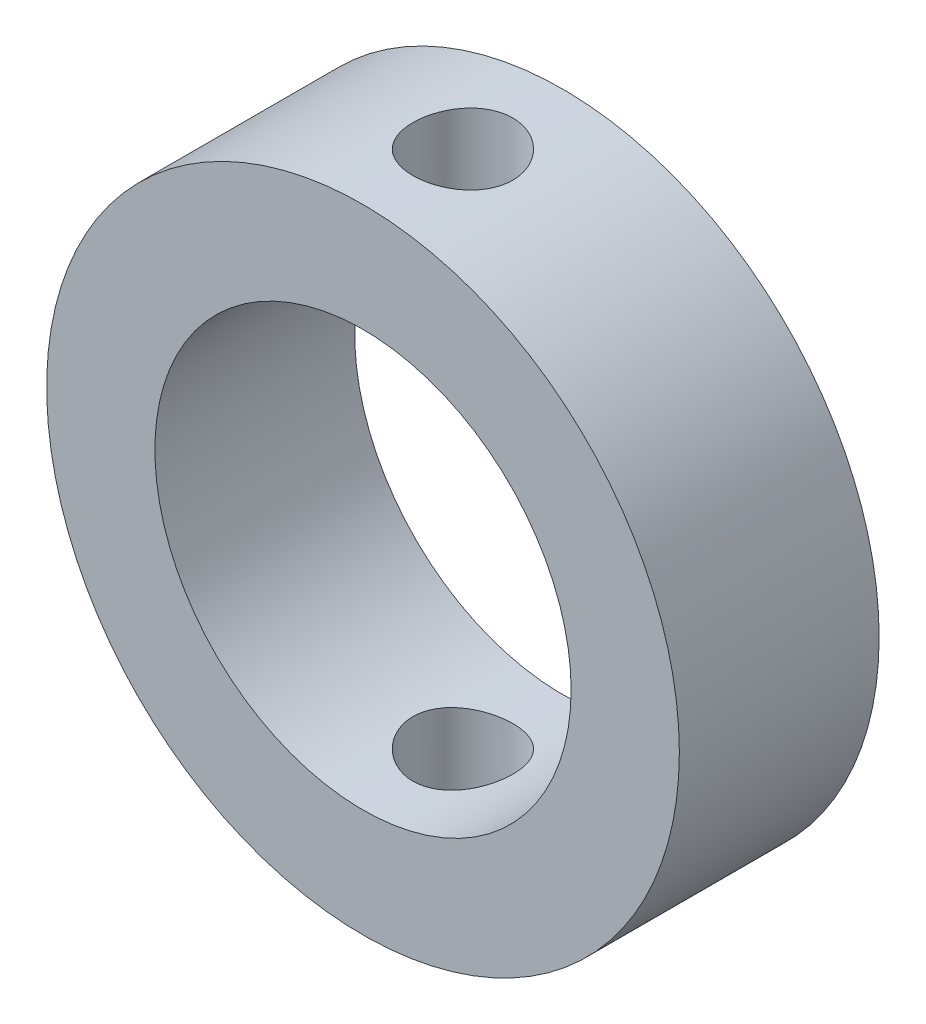
SolidWorks part; units mm, degrees
material "Plain Carbon Steel"
ref_plane "Front Plane" through (0, 0, 0) normal (0, 0, 1) x (1, 0, 0)
ref_plane "Top Plane" through (0, 0, 0) normal (0, 1, 0) x (1, 0, 0)
ref_plane "Right Plane" through (0, 0, 0) normal (1, 0, 0) x (0, 0, -1)
sketch "Collar Ring Sketch" plane through (0, 0, 0) normal (0, 0, 1) x (1, 0, 0)
  circle A0 centre (0, 0) radius 19
  circle A1 centre (0, 0) radius 12.5
  dimension "D1" = 38
  dimension "D2" = 25
extrude "Collar Ring Ø38xØ25" add sketch "Collar Ring Sketch" along normal blind 12
sketch "Cross Hole Sketch" plane through (0, 0, 0) normal (0, 1, 0) x (1, 0, 0)
  line L0 (0, 7.5665) -> (0, -15.6469) construction
  line L1 (19, 0) -> (-19, 0) construction
  circle A0 centre (0, -6) radius 3
  dimension "D1" = 6
  dimension "D2" = 6
extrude "Cross Hole Ø6" cut sketch "Cross Hole Sketch" against normal through all both and the other way through all
